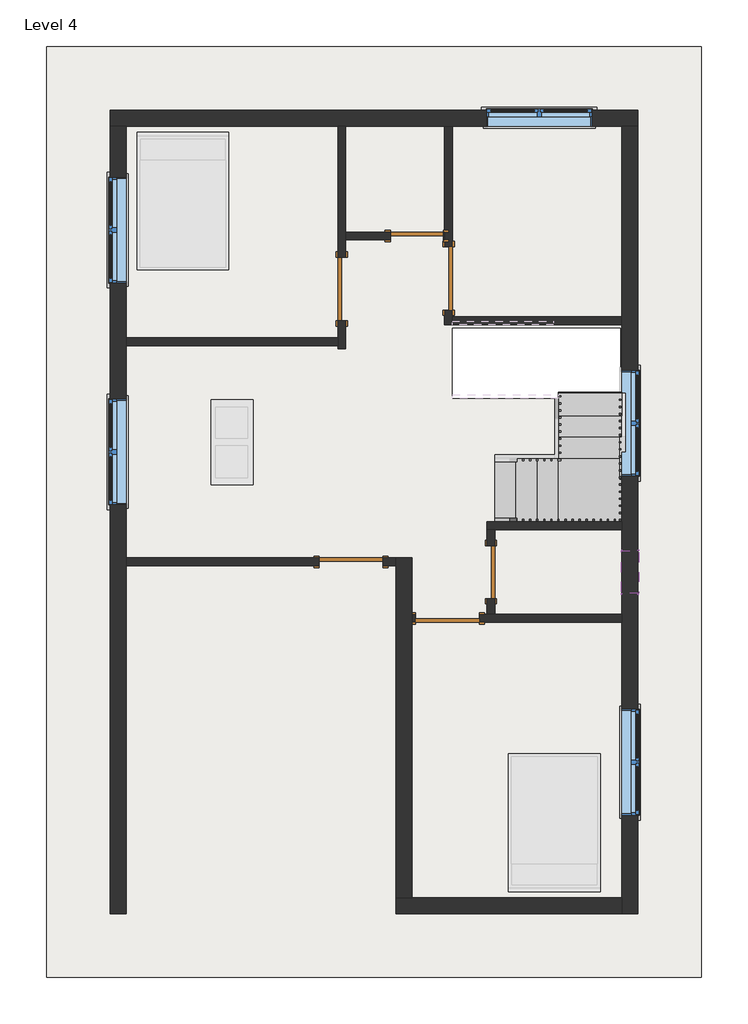
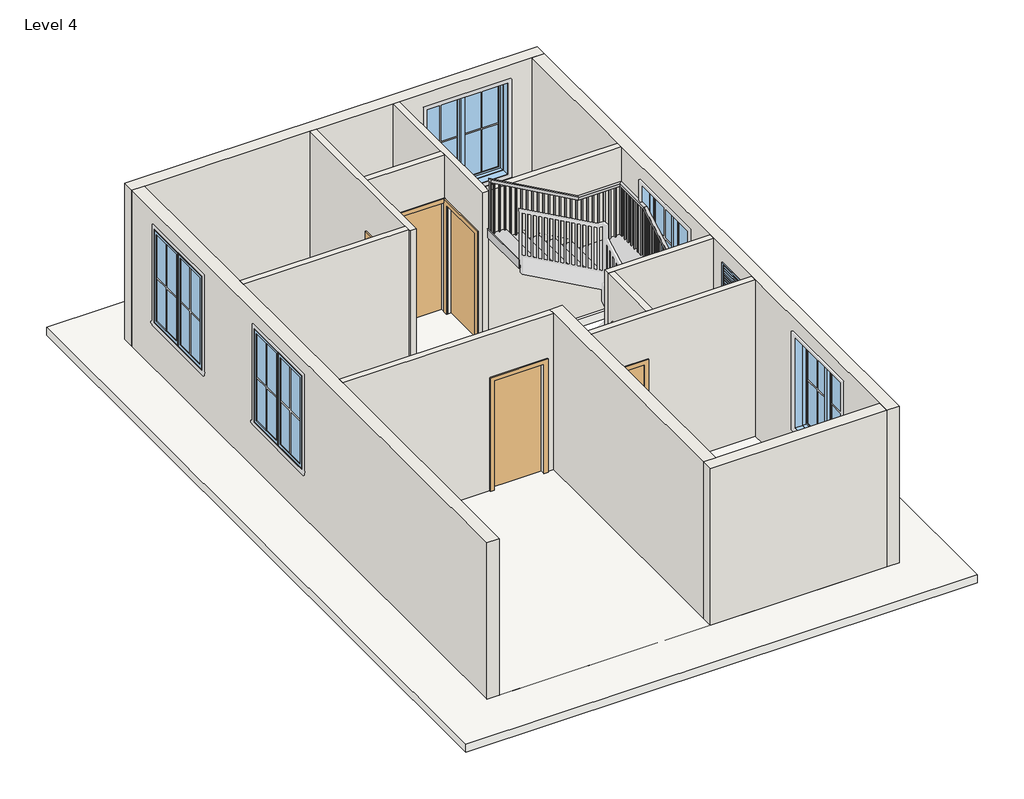
# One storey, part 1 of 2: 14 walls, 6 doors, 6 windows, 1 railing, 1 roof, 1 slab, 1 stair flight.
# Revit data of these elements (continued)
# Element 27 (IfcWindow, "Window-Casement-Double : WIN 5'")
#   Mark = "15"
#   Window Inset = 0' - 0"
#   Interior Wall Closure = 0' - 2 1/4"
#   Frame Extension = 0' - 0 1/4"
#   Exterior Wall Closure = 0' - 1 1/4"
#   Interior Trim Visibility = yes
#   Exterior Trim Visibility = yes
#   Phase Created = New Construction
#   Materials on its faces: "Wood - Stained", "Glass", "Clad - White"
# Element 28 (IfcWindow, "Window-Casement-Double : WIN 5'")
#   Mark = "16"
#   Window Inset = 0' - 0"
#   Interior Wall Closure = 0' - 2 1/4"
#   Frame Extension = 0' - 0 1/4"
#   Exterior Wall Closure = 0' - 1 1/4"
#   Interior Trim Visibility = yes
#   Exterior Trim Visibility = yes
#   Phase Created = New Construction
#   Materials on its faces: "Wood - Stained", "Glass", "Clad - White"
# Element 29 (IfcWindow, "Window-Casement-Double : WIN 5'")
#   Mark = "17"
#   Window Inset = 0' - 0"
#   Interior Wall Closure = 0' - 2 1/4"
#   Frame Extension = 0' - 0 1/4"
#   Exterior Wall Closure = 0' - 1 1/4"
#   Interior Trim Visibility = yes
#   Exterior Trim Visibility = yes
#   Phase Created = New Construction
#   Materials on its faces: "Wood - Stained", "Glass", "Clad - White"
# Element 30 (IfcWindow, "Window-Louvers : 24\" x 24\"")
#   Mark = "18"
#   Blade Width = 1' - 10 1/2"
#   Phase Created = New Construction
#   Materials on its faces: "Birch"
# Materials
#   "Door - Panel": class "Wood", colour RGB 210 159 95, transparency 0, Cost = 0
#   "Door - Frame": colour RGB 118 70 51, transparency 0, Cost = 0
#   "Wood - Stained": class "Wood", colour RGB 224 178 126, transparency 0, Cost = 0
#   "Glass": class "Glass", colour RGB 0 128 192, transparency 0.75, Description = "Soda Lime Glass", Cost = 0
#   "Clad - White": class "Wood", colour RGB 242 242 238, transparency 0, Cost = 0
#   "Birch": class "Wood", colour RGB 224 178 126, transparency 0, Description = "Betula Alleghaniensis", Cost = 0
#   "Default Roof": colour RGB 88 101 114, transparency 0, Cost = 0
#   "Default Floor": colour RGB 128 128 128, transparency 0, Cost = 0
#   "Default Wall": colour RGB 128 128 128, transparency 0, Cost = 0
#   "Copper": class "Metal", colour RGB 0 0 0, transparency 0, Description = "Copper, matte finish", Cost = 0
